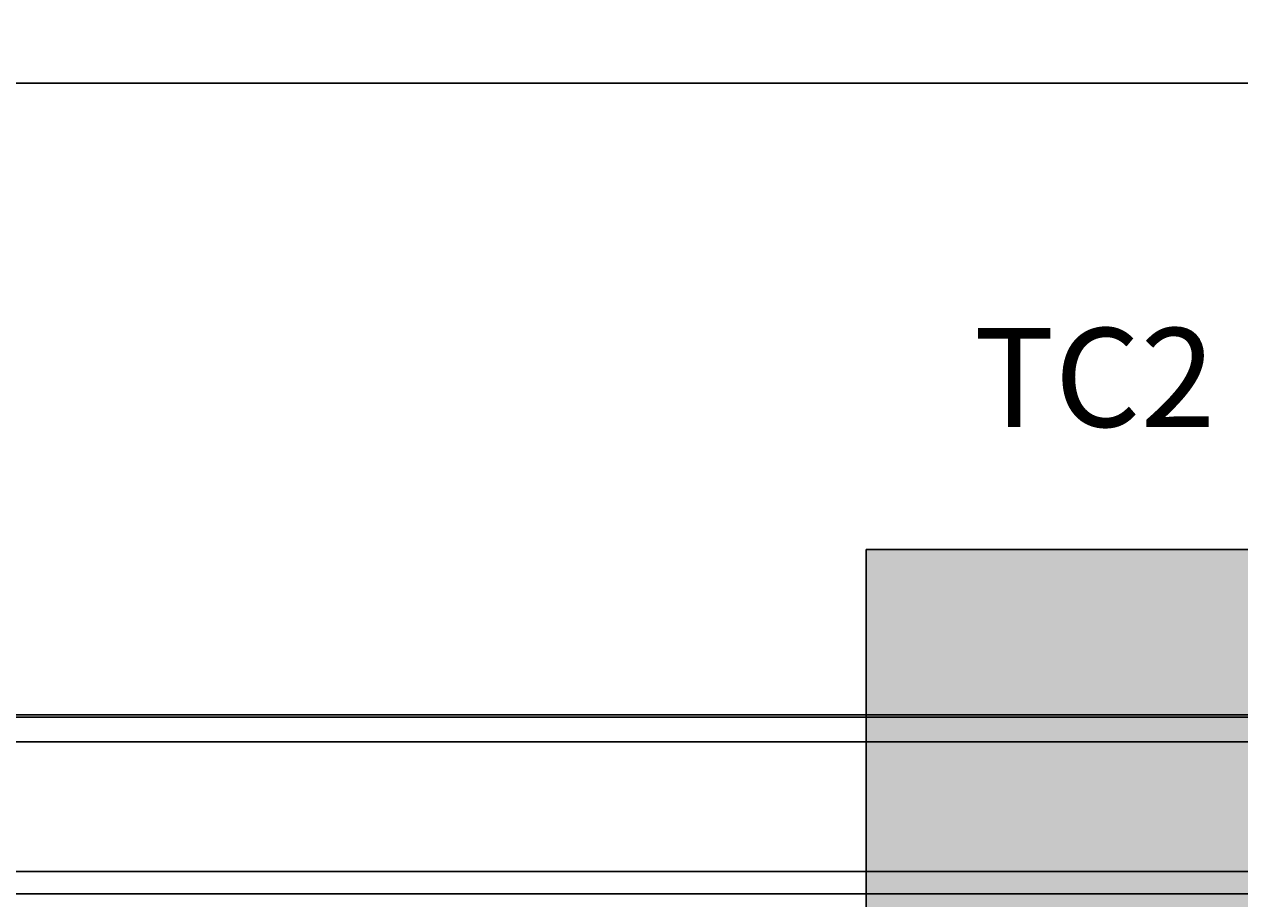
# Model space of a CAD drawing. Units: inches. Extents: x 35362 to 73946, y 43607 to 67532.
# Tile 13 of 134: x 43509 to 46225, y 48909 to 50863. Entities that reach past the tile are written whole.
import ezdxf

# ---------------------------------------------------------------- set-up
doc = ezdxf.new("R2010")
doc.units = ezdxf.units.IN
doc.header["$MEASUREMENT"] = 0
for name, color, linetype, lineweight in [('A-ANNO-DIMS', 2, 'Continuous', 18), ('E-ANNO-TEXT', 5, 'Continuous', 18), ('E-SYMB', 1, 'Continuous', 25), ('E-SYMB-PATT', 1, 'Continuous', 13), ('E-WIRE', 3, 'Continuous', 25)]:
    doc.layers.add(name, color=color, linetype=linetype, lineweight=lineweight)
doc.styles.get("Standard").update_dxf_attribs({"font": 'arial.ttf'})
doc.dimstyles.get("Standard").update_dxf_attribs({"dimtxt": 0.18, "dimasz": 0.18, "dimexe": 0.18, "dimexo": 0.0625, "dimgap": 0.09, "dimtad": 0, "dimtih": 1, "dimtoh": 1, "dimdec": 4, "dimzin": 0, "dimdsep": 46, "dimtxsty": 'Standard', "dimcen": 0.09, "dimadec": 0, "dimazin": 0, "dimtfac": 1, "dimtdec": 4, "dimtofl": 0, "dimtmove": 0, "dimatfit": 3, "dimfxl": 1, "dimtolj": 1, "dimtzin": 0, "dimarcsym": 0})

# ---------------------------------------------------------------- blocks, each defined once
blk = doc.blocks.new('*D40')
at = {"layer": 'A-ANNO-DIMS', "color": 0, "lineweight": -2, "transparency": 16777216}
for p, q in [((56873.5, 53351.5), (35361.8, 53351.5)), ((35361.9, 53351.3), (35361.9, 51333.3)), ((35361.9, 49314.8), (35361.9, 51332.9)), ((51806.5, 49314.7), (35361.8, 49314.7))]:
    blk.add_line(p, q, dxfattribs=at)
at = {"layer": 'A-ANNO-DIMS', "color": 0, "transparency": 16777216}
for points in [[(35361.9, 53351.3), (35362, 53351.3), (35361.9, 53351.5)], [(35361.9, 49314.8), (35362, 49314.8), (35361.9, 49314.7)]]:
    blk.add_solid(points, dxfattribs=at)
at = {"layer": 'Defpoints', "color": 0, "transparency": 16777216}
for p in [(35361.9, 53351.5), (56873.6, 53351.5), (51806.5, 49314.7)]:
    blk.add_point(p, dxfattribs=at)
at = {"layer": 'A-ANNO-DIMS', "color": 0, "transparency": 16777216, "insert": (35361.9, 51333.1), "char_height": 0.18, "attachment_point": 5}
blk.add_mtext('\\A1;4036.9', dxfattribs=at)
blk = doc.blocks.new('*D67')
at = {"layer": 'A-ANNO-DIMS', "color": 0, "lineweight": -2, "transparency": 16777216}
for p, q in [((56873.5, 53351.5), (35361.8, 53351.5)), ((35361.9, 53351.3), (35361.9, 49400.9)), ((35361.9, 45450.1), (35361.9, 49400.5)), ((53793.6, 45449.9), (35361.8, 45449.9))]:
    blk.add_line(p, q, dxfattribs=at)
at = {"layer": 'A-ANNO-DIMS', "color": 0, "transparency": 16777216}
for points in [[(35361.9, 53351.3), (35362, 53351.3), (35361.9, 53351.5)], [(35361.9, 45450.1), (35362, 45450.1), (35361.9, 45449.9)]]:
    blk.add_solid(points, dxfattribs=at)
at = {"layer": 'Defpoints', "color": 0, "transparency": 16777216}
for p in [(35361.9, 53351.5), (56873.6, 53351.5), (53793.6, 45449.9)]:
    blk.add_point(p, dxfattribs=at)
at = {"layer": 'A-ANNO-DIMS', "color": 0, "transparency": 16777216, "insert": (35361.9, 49400.7), "char_height": 0.18, "attachment_point": 5}
blk.add_mtext('\\A1;7901.6', dxfattribs=at)
blk = doc.blocks.new('*D84')
at = {"layer": 'A-ANNO-DIMS', "color": 0, "lineweight": -2, "transparency": 16777216}
for p, q in [((55540.2, 49259.9), (35361.8, 49259.9)), ((35361.9, 49259.8), (35361.9, 49115.1)), ((35361.9, 48970.2), (35361.9, 49114.8)), ((55540.2, 48970), (35361.8, 48970))]:
    blk.add_line(p, q, dxfattribs=at)
at = {"layer": 'A-ANNO-DIMS', "color": 0, "transparency": 16777216}
for points in [[(35361.9, 49259.8), (35362, 49259.8), (35361.9, 49259.9)], [(35361.9, 48970.2), (35362, 48970.2), (35361.9, 48970)]]:
    blk.add_solid(points, dxfattribs=at)
at = {"layer": 'Defpoints', "color": 0, "transparency": 16777216}
for p in [(35361.9, 49259.9), (55540.3, 49259.9), (55540.3, 48970)]:
    blk.add_point(p, dxfattribs=at)
at = {"layer": 'A-ANNO-DIMS', "color": 0, "transparency": 16777216, "insert": (35361.9, 49115), "char_height": 0.18, "attachment_point": 5}
blk.add_mtext('\\A1;289.96', dxfattribs=at)
blk = doc.blocks.new('*D86')
at = {"layer": 'A-ANNO-DIMS', "color": 0, "lineweight": -2, "transparency": 16777216}
for p, q in [((51285.5, 49320.1), (35361.8, 49320.1)), ((35361.9, 49319.9), (35361.9, 49120.3)), ((35361.9, 48920.3), (35361.9, 49119.9)), ((51285.5, 48920.1), (35361.8, 48920.1))]:
    blk.add_line(p, q, dxfattribs=at)
at = {"layer": 'A-ANNO-DIMS', "color": 0, "transparency": 16777216}
for points in [[(35361.9, 49319.9), (35362, 49319.9), (35361.9, 49320.1)], [(35361.9, 48920.3), (35362, 48920.3), (35361.9, 48920.1)]]:
    blk.add_solid(points, dxfattribs=at)
at = {"layer": 'Defpoints', "color": 0, "transparency": 16777216}
for p in [(35361.9, 49320.1), (51285.6, 49320.1), (51285.6, 48920.1)]:
    blk.add_point(p, dxfattribs=at)
at = {"layer": 'A-ANNO-DIMS', "color": 0, "transparency": 16777216, "insert": (35361.9, 49120.1), "char_height": 0.18, "attachment_point": 5}
blk.add_mtext('\\A1;400.0', dxfattribs=at)

msp = doc.modelspace()

# ---------------------------------------------------------------- hatches: boundary and pattern name
at = {"layer": 'E-SYMB-PATT'}
h = msp.add_hatch(color=256, dxfattribs=at)
h.dxf.hatch_style = 1
h.paths.add_polyline_path([(48163.038, 49689.843), (45390.147, 49689.843), (45390.147, 46919.381), (48163.038, 46919.381)])

# ---------------------------------------------------------------- linework, layer by layer
at = {"layer": 'E-SYMB'}
msp.add_lwpolyline([(45390.147, 49689.843), (48163.038, 49689.843), (48163.038, 46919.381), (45390.147, 46919.381)], close=True, dxfattribs=at)
at = {"layer": 'E-WIRE'}
msp.add_line((38575.774, 50731.821), (54718.752, 50731.821), dxfattribs=at)

# ---------------------------------------------------------------- texts
at = {"layer": 'E-ANNO-TEXT'}
msp.add_text('TC2', height=220.866, dxfattribs=at).set_placement((45630.34, 49963.616))

# ---------------------------------------------------------------- dimensions: what is measured, and where the dimension line sits
at = {"layer": 'A-ANNO-DIMS'}
for base, p1, p2, override, picture, middle in [((35361.949, 53351.529), (51806.517, 49314.669), (56873.602, 53351.529), {"dimdec": 1, "dimlfac": 1, "dimrnd": 0, "dimzin": 0, "dimdsep": 46, "dimlunit": 2}, '*D40', (35361.949, 51333.099)), ((35361.949, 53351.529), (53793.638, 45449.894), (56873.602, 53351.529), {"dimdec": 1, "dimlfac": 1, "dimrnd": 0, "dimzin": 0, "dimdsep": 46, "dimlunit": 2}, '*D67', (35361.949, 49400.712)), ((35361.949, 49320.079), (51285.595, 48920.079), (51285.595, 49320.079), {"dimdec": 1, "dimlfac": 1, "dimrnd": 0, "dimzin": 0, "dimdsep": 46, "dimlunit": 2}, '*D86', (35361.949, 49120.079)), ((35361.9491, 49259.9353), (55540.2972, 48969.9796), (55540.2972, 49259.9353), {"dimdec": 2, "dimlfac": 1, "dimrnd": 0, "dimzin": 0, "dimdsep": 46, "dimlunit": 2}, '*D84', (35361.9491, 49114.9575))]:
    dim = msp.add_linear_dim(base=base, p1=p1, p2=p2, angle=90, dimstyle='Standard', override=override, dxfattribs=at)
    dim.commit()
    dim.dimension.update_dxf_attribs({"geometry": picture, "text_midpoint": middle})

doc.saveas('drawing.dxf')
